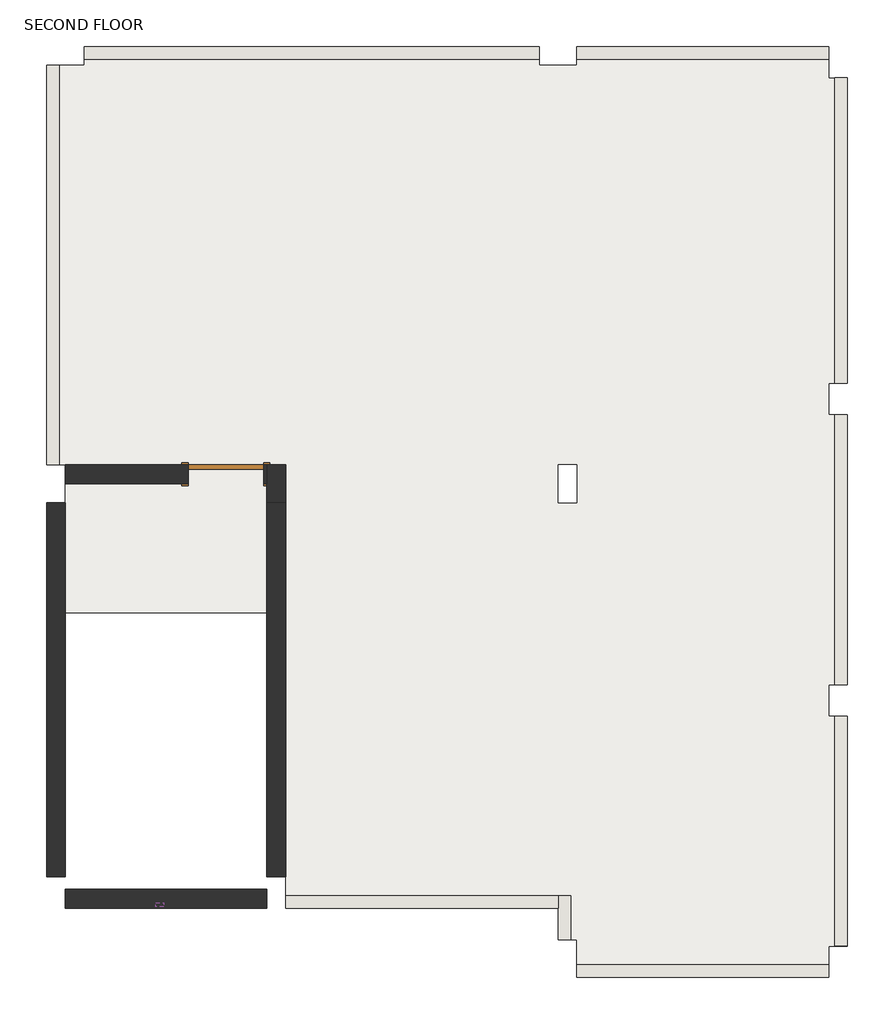
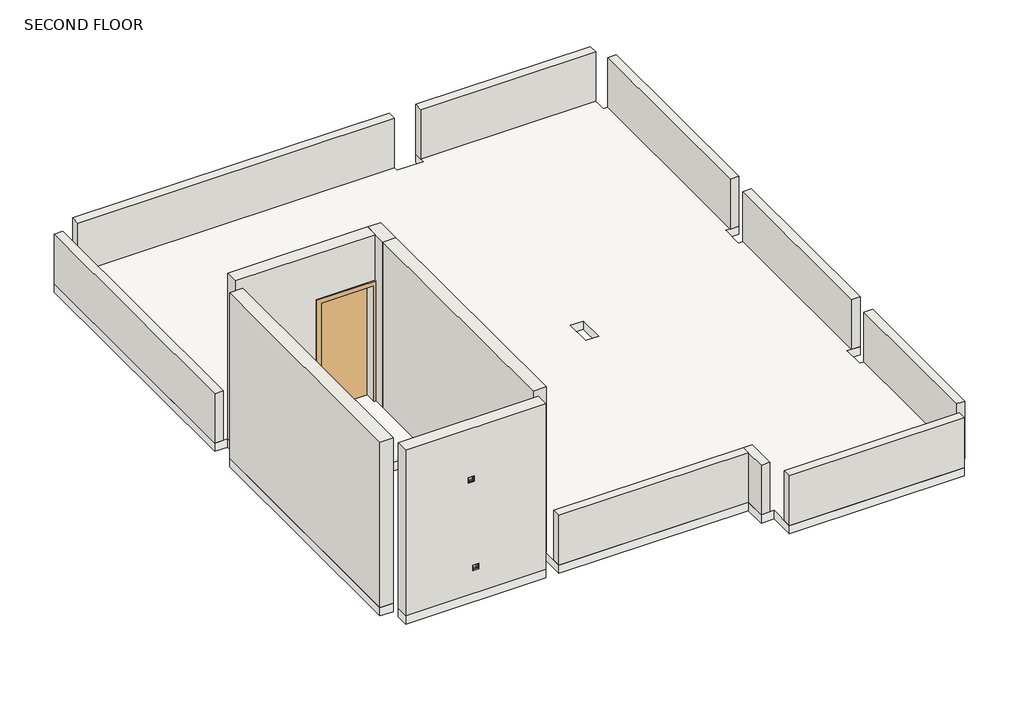
# One storey: 14 walls, 2 light fixtures, 1 door, 1 slab.
"""IFC4 building model written with IfcOpenShell, lengths in millimetres."""

from ifc_helpers import new_model, si_unit, frame, origin, place, context, project, spatial, polyline, outline, extrude, faceted_brep, transform, mapped, element, save
from components import single_flush_3_x7_0ca8825f, light_fixture_da35b629

model = new_model("IFC4")

# Units and contexts
model_context = context("Model", 3, world=origin())
ifc_project = project(units=[si_unit("LENGTHUNIT", "METRE", prefix="MILLI")], contexts=[model_context])

# Site, building, storey
site = spatial("IfcSite", under=ifc_project)
building = spatial("IfcBuilding", under=site)
storey = spatial("IfcBuildingStorey", under=building, Name="SECOND FLOOR", Elevation=6400.8)

# Door
placement = place(None, origin())
single_flush_3_x7_shape = single_flush_3_x7_0ca8825f(model_context)
element("IfcDoor", 1, ObjectType="Single-Flush : 3'X7'", at=placement, inside=storey, context=model_context, shape_type="MappedRepresentation", body=[
    mapped(single_flush_3_x7_shape, transform((-10719.7209734, 3706.1170657, 6400.8), x_axis=(1.0, 0.0, 0.0), y_axis=(0.0, 1.0, 0.0), z_axis=(0.0, 0.0, 1.0))),
])

# Light fixtures
light_fixture_shape = light_fixture_da35b629(model_context)
element("IfcLightFixture", 2, at=placement, inside=storey, context=model_context, shape_type="MappedRepresentation", body=[
    mapped(light_fixture_shape, transform((-11556.1766361, -1437.3829343, 6510.9998908), x_axis=(-1.0, 0.0, 0.0), y_axis=(0.0, -1.0, 0.0), z_axis=(0.0, 0.0, 1.0))),
])
element("IfcLightFixture", 3, at=placement, inside=storey, context=model_context, shape_type="MappedRepresentation", body=[
    mapped(light_fixture_shape, transform((-11479.9766361, -1437.3829343, 4875.0652515), x_axis=(-1.0, 0.0, 0.0), y_axis=(0.0, -1.0, 0.0), z_axis=(0.0, 0.0, 1.0))),
])

# Slab
element("IfcSlab", 4, ObjectType="6\"", at=placement, inside=storey, context=model_context, shape_type="SweptSolid", body=[
    extrude(outline(polyline([(-12662.8209734, -1323.0829343), (-10224.4209734, -1323.0829343), (-10224.4209734, -1551.6829343), (-12662.8209734, -1551.6829343), (-12662.8209734, -1323.0829343)])), frame((0.0, 0.0, 6248.4), z_axis=(0.0, 0.0, 1.0), x_axis=(1.0, 0.0, 0.0)), (0.0, 0.0, 1.0), 152.4),
    extrude(outline(polyline([(-10224.4209734, 2029.7170657), (-12662.8209734, 2029.7170657), (-12662.8209734, -1170.6829343), (-12891.4209734, -1170.6829343), (-12891.4209734, 3363.2170657), (-12662.8209734, 3363.2170657), (-12662.8209734, 3820.4170657), (-12891.4209734, 3820.4170657), (-12891.4209734, 8659.1170657), (-12434.2209734, 8659.1170657), (-12434.2209734, 8887.7170657), (-6922.4209734, 8887.7170657), (-6922.4209734, 8659.1170657), (-6465.2209734, 8659.1170657), (-6465.2209734, 8887.7170657), (-3417.2209734, 8887.7170657), (-3417.2209734, 8506.7170657), (-3188.6209734, 8506.7170657), (-3188.6209734, 4811.0170657), (-3417.2209734, 4811.0170657), (-3417.2209734, 4430.0170657), (-3188.6209734, 4430.0170657), (-3188.6209734, 1153.4170657), (-3417.2209734, 1153.4170657), (-3417.2209734, 772.4170657), (-3188.6209734, 772.4170657), (-3188.6209734, -2008.8829343), (-3417.2209734, -2008.8829343), (-3417.2209734, -2389.8829343), (-6465.2209734, -2389.8829343), (-6465.2209734, -1932.6829343), (-6693.8209734, -1932.6829343), (-6693.8209734, -1551.6829343), (-9995.8209734, -1551.6829343), (-9995.8209734, -1170.6829343), (-10224.4209734, -1170.6829343), (-10224.4209734, 2029.7170657)]), holes=[polyline([(-6693.8209734, 3820.4170657), (-6693.8209734, 3363.2170657), (-6465.2209734, 3363.2170657), (-6465.2209734, 3820.4170657), (-6693.8209734, 3820.4170657)])]), frame((0.0, 0.0, 6248.4), z_axis=(0.0, 0.0, 1.0), x_axis=(1.0, 0.0, 0.0)), (0.0, 0.0, 1.0), 152.4),
])

# Walls
element("IfcWall", 5, ObjectType="6\"", at=placement, inside=storey, context=model_context, shape_type="SweptSolid", body=[
    extrude(outline(polyline([(-12739.0209734, 8659.1170657), (-12739.0209734, 3820.4170657), (-12891.4209734, 3820.4170657), (-12891.4209734, 8659.1170657), (-12739.0209734, 8659.1170657)])), frame((0.0, 0.0, 6400.8), z_axis=(0.0, 0.0, 1.0), x_axis=(1.0, 0.0, 0.0)), (0.0, 0.0, 1.0), 914.4),
])
element("IfcWall", 6, ObjectType="6\"", at=placement, inside=storey, context=model_context, shape_type="SweptSolid", body=[
    extrude(outline(polyline([(-6922.4209734, 8735.3170657), (-12434.2209734, 8735.3170657), (-12434.2209734, 8887.7170657), (-6922.4209734, 8887.7170657), (-6922.4209734, 8735.3170657)])), frame((0.0, 0.0, 6400.8), z_axis=(0.0, 0.0, 1.0), x_axis=(1.0, 0.0, 0.0)), (0.0, 0.0, 1.0), 914.4),
])
element("IfcWall", 7, ObjectType="6\"", at=placement, inside=storey, context=model_context, shape_type="SweptSolid", body=[
    extrude(outline(polyline([(-3417.2209734, 8735.3170657), (-6465.2209734, 8735.3170657), (-6465.2209734, 8887.7170657), (-3417.2209734, 8887.7170657), (-3417.2209734, 8735.3170657)])), frame((0.0, 0.0, 6400.8), z_axis=(0.0, 0.0, 1.0), x_axis=(1.0, 0.0, 0.0)), (0.0, 0.0, 1.0), 914.4),
])
element("IfcWall", 8, ObjectType="6\"", at=placement, inside=storey, context=model_context, shape_type="SweptSolid", body=[
    extrude(outline(polyline([(-3341.0209734, 4811.0170657), (-3341.0209734, 8506.7170657), (-3188.6209734, 8506.7170657), (-3188.6209734, 4811.0170657), (-3341.0209734, 4811.0170657)])), frame((0.0, 0.0, 6400.8), z_axis=(0.0, 0.0, 1.0), x_axis=(1.0, 0.0, 0.0)), (0.0, 0.0, 1.0), 914.4),
])
element("IfcWall", 9, ObjectType="6\"", at=placement, inside=storey, context=model_context, shape_type="SweptSolid", body=[
    extrude(outline(polyline([(-3341.0209734, 1153.4170657), (-3341.0209734, 4430.0170657), (-3188.6209734, 4430.0170657), (-3188.6209734, 1153.4170657), (-3341.0209734, 1153.4170657)])), frame((0.0, 0.0, 6400.8), z_axis=(0.0, 0.0, 1.0), x_axis=(1.0, 0.0, 0.0)), (0.0, 0.0, 1.0), 914.4),
])
element("IfcWall", 10, ObjectType="6\"", at=placement, inside=storey, context=model_context, shape_type="SweptSolid", body=[
    extrude(outline(polyline([(-3341.0209734, -2008.8829343), (-3341.0209734, 772.4170657), (-3188.6209734, 772.4170657), (-3188.6209734, -2008.8829343), (-3341.0209734, -2008.8829343)])), frame((0.0, 0.0, 6400.8), z_axis=(0.0, 0.0, 1.0), x_axis=(1.0, 0.0, 0.0)), (0.0, 0.0, 1.0), 914.4),
])
element("IfcWall", 11, ObjectType="6\"", at=placement, inside=storey, context=model_context, shape_type="SweptSolid", body=[
    extrude(outline(polyline([(-6465.2209734, -2237.4829343), (-3417.2209734, -2237.4829343), (-3417.2209734, -2389.8829343), (-6465.2209734, -2389.8829343), (-6465.2209734, -2237.4829343)])), frame((0.0, 0.0, 6400.8), z_axis=(0.0, 0.0, 1.0), x_axis=(1.0, 0.0, 0.0)), (0.0, 0.0, 1.0), 914.4),
])
element("IfcWall", 12, ObjectType="6\"", at=placement, inside=storey, context=model_context, shape_type="SweptSolid", body=[
    extrude(outline(polyline([(-6693.8209734, -1551.6829343), (-9995.8209734, -1551.6829343), (-9995.8209734, -1399.2829343), (-6693.8209734, -1399.2829343), (-6693.8209734, -1551.6829343)])), frame((0.0, 0.0, 6400.8), z_axis=(0.0, 0.0, 1.0), x_axis=(1.0, 0.0, 0.0)), (0.0, 0.0, 1.0), 914.4),
])
element("IfcWall", 13, ObjectType="6\"", at=placement, inside=storey, context=model_context, shape_type="Brep", body=[
    faceted_brep([(-6693.8209734, -1399.2829343, 6400.8), (-6693.8209734, -1551.6829343, 6400.8), (-6693.8209734, -1932.6829343, 6400.8), (-6693.8209734, -1932.6829343, 7315.2), (-6693.8209734, -1551.6829343, 7315.2), (-6693.8209734, -1399.2829343, 7315.2), (-6541.4209734, -1399.2829343, 6400.8), (-6541.4209734, -1399.2829343, 7315.2), (-6541.4209734, -1932.6829343, 7315.2), (-6541.4209734, -1932.6829343, 6400.8)], [[[0, 1, 2, 3, 4, 5]], [[6, 7, 8, 9]], [[2, 1, 0, 6, 9]], [[3, 2, 9, 8]], [[5, 4, 3, 8, 7]], [[0, 5, 7, 6]]]),
])
element("IfcWall", 14, ObjectType="9\"", at=placement, inside=storey, context=model_context, shape_type="SweptSolid", body=[
    extrude(outline(polyline([(-12662.8209734, 3363.2170657), (-12662.8209734, -1170.6829343), (-12891.4209734, -1170.6829343), (-12891.4209734, 3363.2170657), (-12662.8209734, 3363.2170657)])), frame((0.0, 0.0, 6400.8), z_axis=(0.0, 0.0, 1.0), x_axis=(1.0, 0.0, 0.0)), (0.0, 0.0, 1.0), 3048.0),
])
element("IfcWall", 15, ObjectType="9\"", at=placement, inside=storey, context=model_context, shape_type="SweptSolid", body=[
    extrude(outline(polyline([(-9995.8209734, 3363.2170657), (-9995.8209734, -1170.6829343), (-10224.4209734, -1170.6829343), (-10224.4209734, 3363.2170657), (-9995.8209734, 3363.2170657)])), frame((0.0, 0.0, 6400.8), z_axis=(0.0, 0.0, 1.0), x_axis=(1.0, 0.0, 0.0)), (0.0, 0.0, 1.0), 3048.0),
])
element("IfcWall", 16, ObjectType="9\"", at=placement, inside=storey, context=model_context, shape_type="SweptSolid", body=[
    extrude(outline(polyline([(8534.4, -10262.5209734), (6400.8, -10262.5209734), (6400.8, -10224.4209734), (9448.8, -10224.4209734), (9448.8, -12662.8209734), (6400.8, -12662.8209734), (6400.8, -11176.9209734), (8534.4, -11176.9209734), (8534.4, -10262.5209734)])), frame((0.0, 3591.8170657, 0.0), z_axis=(0.0, 1.0, 0.0), x_axis=(0.0, 0.0, 1.0)), (0.0, 0.0, 1.0), 228.6),
])
element("IfcWall", 17, ObjectType="9\"", at=placement, inside=storey, context=model_context, shape_type="Brep", body=[
    faceted_brep([(-10224.4209734, 3820.4170657, 6400.8), (-10224.4209734, 3591.8170657, 6400.8), (-10224.4209734, 3363.2170657, 6400.8), (-10224.4209734, 3363.2170657, 9448.8), (-10224.4209734, 3591.8170657, 9448.8), (-10224.4209734, 3820.4170657, 9448.8), (-9995.8209734, 3820.4170657, 6400.8), (-9995.8209734, 3820.4170657, 9448.8), (-9995.8209734, 3363.2170657, 9448.8), (-9995.8209734, 3363.2170657, 6400.8)], [[[0, 1, 2, 3, 4, 5]], [[6, 7, 8, 9]], [[2, 1, 0, 6, 9]], [[3, 2, 9, 8]], [[5, 4, 3, 8, 7]], [[0, 5, 7, 6]]]),
])
element("IfcWall", 18, ObjectType="9\"", at=placement, inside=storey, context=model_context, shape_type="SweptSolid", body=[
    extrude(outline(polyline([(6400.8, -12662.8209734), (6400.8, -10224.4209734), (9448.8, -10224.4209734), (9448.8, -12662.8209734), (6400.8, -12662.8209734)]), holes=[polyline([(8560.9998908, -11469.8209734), (8460.9998908, -11469.8209734), (8460.9998908, -11569.8209734), (8560.9998908, -11569.8209734), (8560.9998908, -11469.8209734)]), polyline([(6925.0652515, -11393.6209734), (6825.0652515, -11393.6209734), (6825.0652515, -11493.6209734), (6925.0652515, -11493.6209734), (6925.0652515, -11393.6209734)])]), frame((0.0, -1551.6829343, 0.0), z_axis=(0.0, 1.0, 0.0), x_axis=(0.0, 0.0, 1.0)), (0.0, 0.0, 1.0), 228.6),
])

save(model, "model.ifc")

# Revit data of these elements
# Type "Single-Flush : 3'X7'"
#   Type Mark = "8"
#   Construction Type Id = "MDOOR"
#   Assembly Code = "C1020"
#   Analytic Construction = "Metal"
#   Thickness = 0' - 2"
#   Heat Transfer Coefficient (U) = 0.651978 BTU/(h·ft²·°F)
#   Height = 7' - 0"
#   Trim Projection Ext = 0' - 1"
#   Trim Projection Int = 0' - 1"
#   Trim Width = 0' - 3"
#   Width = 3' - 0"
#   Define Thermal Properties by = 1
#   Door Material = Door - Panel
#   Frame Material = Door - Frame
#   Visual Light Transmittance = 0
#   Solar Heat Gain Coefficient = 0
#   Function = (empty or 0)
#   Wall Closure = (empty or 0)
# Type
#   rahmen dicke = 0' - 0.98819"
#   rahmen breite(okvir) = 0' - 0.55118"
#   rahmen breite = 0' - 1.9685"
#   glas dicke = 0' - 0.82349"
#   abstand von wand (lichtquelle) = 0' - 2.76378"
#   Wattage = 20.16 W
#   Emit from Circle Diameter = 0' - 4.31496"
#   built-in parameter 1150110 = 1 (stored number, unit not read)
#   built-in parameter 1114217 = 1 (stored number, unit not read)
#   built-in parameter 1150109 = 1 (stored number, unit not read)
#   built-in parameter 1150113 = 1 (stored number, unit not read)
#   Lumens = 2994.61 lm
#   built-in parameter 1150115 = 1 (stored number, unit not read)
#   built-in parameter 1150105 = 953.213 (stored number, unit not read)
#   Light Source Symbol Size = 2' - 0"
#   built-in parameter 1150112 = 1 (stored number, unit not read)
#   built-in parameter 1150114 = 1 (stored number, unit not read)
#   built-in parameter 1150107 = 3000 (stored number, unit not read)
#   built-in parameter 1150106 = 9.53213 (stored number, unit not read)
#   built-in parameter 1150104 = 13.8 (stored number, unit not read)
#   built-in parameter 1114218 = 1 (stored number, unit not read)
#   built-in parameter 1150133 = 10 (stored number, unit not read)
#   Emit Shape Visible in Rendering = yes
#   Color Filter = 16744448
#   rahmen material = rahmen material
#   glass material = glas material
#   Dimming Lamp Color Temperature Shift = (empty or 0)
#   Default Elevation = 0
# Type "6\""
#   Assembly Code = "B1010"
#   Function = 0
#   Layers, outside or top first: 0' - 6" no material (function 1)
# Type "6\""
#   Assembly Code = "B2010"
#   Layers, outside or top first: 0' - 6" no material (function 1)
# Type "9\""
#   Assembly Code = "B2010"
#   Layers, outside or top first: 0' - 9" no material (function 1)
# Element 1 (IfcDoor, "Single-Flush : 3'X7'")
#   Phase Created = New Construction
#   Materials on its faces: "Door - Frame", "Door - Panel"
# Element 2 (IfcLightFixture)
#   Mark = "1"
#   Phase Created = New Construction
#   Materials on its faces: "rahmen material", "glas material"
# Element 3 (IfcLightFixture)
#   Mark = "2"
#   Phase Created = New Construction
#   Materials on its faces: "rahmen material", "glas material"
# Element 4 (IfcSlab, "6\"")
#   Height Offset From Level = 0' - 0"
#   Phase Created = New Construction
#   Materials on its faces: "Default Floor", "Softwood, Lumber"
# Elements 5, 6, 7, 8, 9, 10 (IfcWall, "6\"")
#   Top Offset = -0' - 6"
#   Base Offset = 0' - 0"
#   Unconnected Height = 3' - 0"
#   wall height = 3' - 0"
#   Phase Created = New Construction
#   Base Constraint = SECOND FLOOR
#   Materials on its faces: "Default Wall", "EIFS, Exterior Insulation"
# Elements 11, 12 (IfcWall, "6\"")
#   Top Offset = -0' - 6"
#   Base Offset = 0' - 0"
#   Unconnected Height = 3' - 0"
#   wall height = 3' - 0"
#   Phase Created = New Construction
#   Base Constraint = SECOND FLOOR
#   Materials on its faces: "Default Wall", "Tile, Porcelain, 4in"
# Element 13 (IfcWall, "6\"")
#   Top Offset = -0' - 6"
#   Base Offset = 0' - 0"
#   Unconnected Height = 3' - 0"
#   wall height = 3' - 0"
#   Phase Created = New Construction
#   Base Constraint = SECOND FLOOR
#   Materials on its faces: "Default Wall"
# Element 14 (IfcWall, "9\"")
#   Top Offset = -0' - 6"
#   Base Offset = 0' - 0"
#   wall height = 10' - 0"
#   Phase Created = New Construction
#   Base Constraint = SECOND FLOOR
#   Top Constraint = ROOF
#   Materials on its faces: "Default Wall", "EIFS, Exterior Insulation"
# Elements 15, 16, 17 (IfcWall, "9\"")
#   Top Offset = -0' - 6"
#   Base Offset = 0' - 0"
#   wall height = 10' - 0"
#   Phase Created = New Construction
#   Base Constraint = SECOND FLOOR
#   Top Constraint = ROOF
#   Materials on its faces: "Default Wall"
# Element 18 (IfcWall, "9\"")
#   Top Offset = -0' - 6"
#   Base Offset = 0' - 0"
#   wall height = 10' - 0"
#   Phase Created = New Construction
#   Base Constraint = SECOND FLOOR
#   Top Constraint = ROOF
#   Materials on its faces: "Default Wall", "Softwood, Lumber"
# Materials
#   "Door - Panel": class "Wood", colour RGB 210 159 95, transparency 0, Cost = 0
#   "Door - Frame": colour RGB 118 70 51, transparency 0, Cost = 0
#   "rahmen material": class "Glas", colour RGB 0 0 255, transparency 0.75
#   "glas material": class "Glas", colour RGB 0 128 192, transparency 0.9
#   "Default Floor": colour RGB 128 128 128, transparency 0, Cost = 0
#   "Softwood, Lumber": class "Wood", colour RGB 223 192 134, transparency 0, Description = "Pinus Echinata", Cost = 0
#   "Default Wall": colour RGB 128 128 128, transparency 0, Cost = 0
#   "EIFS, Exterior Insulation": class "Generic", colour RGB 127 127 127, transparency 0, Description = "EIFS - Exterior Insulation", Cost = 0
#   "Tile, Porcelain, 4in": class "Generic", colour RGB 89 87 158, transparency 0, Description = "Porcelain tile, 4\", white", Cost = 0
